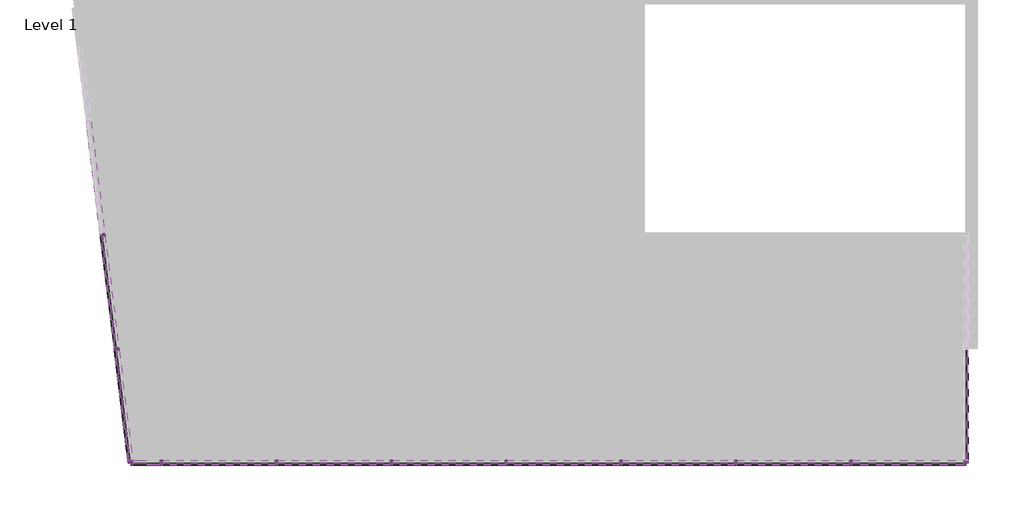
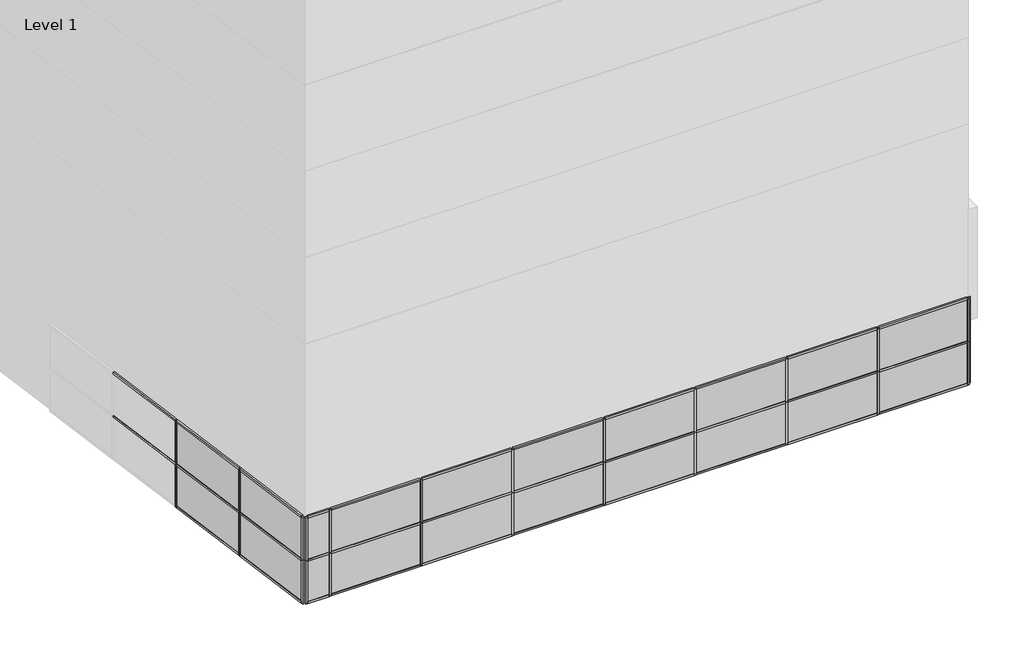
# One storey, part 1 of 2: 60 members, 22 plates.
"""IFC4 building model written with IfcOpenShell, lengths in millimetres."""

from ifc_helpers import new_model, si_unit, origin, place, context, project, spatial, transform, mapped, element, save
from components import member_71c27fd2, member_19d0a4ec, member_8cef0660, member_db480205, member_82905deb, member_4491d118, member_695b83e4, member_0c11e56c, system_panel_glazed_37f15d2e, system_panel_glazed_3620f98e, system_panel_glazed_e46d4b42, system_panel_glazed_2a6c68b7, system_panel_glazed_07b088f8, system_panel_glazed_9d0e0944

model = new_model("IFC4")

# Units and contexts
model_context = context("Model", 3, world=origin())
ifc_project = project(units=[si_unit("LENGTHUNIT", "METRE", prefix="MILLI")], contexts=[model_context])

# Site, building, storey
site = spatial("IfcSite", under=ifc_project)
building = spatial("IfcBuilding", under=site)
storey = spatial("IfcBuildingStorey", under=building, Name="Level 1", Elevation=0.0)

# Members
placement = place(None, origin())
member_shape = member_71c27fd2(model_context)
element("IfcMember", 1, ObjectType="Rectangular Mullion : 2.5\" x 5\" rectangular", at=placement, inside=storey, context=model_context, shape_type="MappedRepresentation", body=[
    mapped(member_shape, transform((-8620.3262186, -3985.3690403, 0.0), x_axis=(0.0, 0.0, -1.0), y_axis=(-0.9925461516413222, -0.12186934340514607, 0.0), z_axis=(-0.12186934340514607, 0.9925461516413222, 0.0))),
])
element("IfcMember", 2, ObjectType="Rectangular Mullion : 2.5\" x 5\" rectangular", at=placement, inside=storey, context=model_context, shape_type="MappedRepresentation", body=[
    mapped(member_shape, transform((10886.265636, -6979.1363705, 0.0), x_axis=(0.0, 0.0, -1.0), y_axis=(0.0, -1.0, 0.0), z_axis=(-1.0, 0.0, 0.0))),
])
element("IfcMember", 3, ObjectType="Rectangular Mullion : 2.5\" x 5\" rectangular", at=placement, inside=storey, context=model_context, shape_type="MappedRepresentation", body=[
    mapped(member_shape, transform((13902.5156363, -6915.6363705, 0.0), x_axis=(0.0, 0.0, -1.0), y_axis=(1.0, 0.0, 0.0), z_axis=(0.0, -1.0, 0.0))),
])
member_2_shape = member_19d0a4ec(model_context)
element("IfcMember", 4, ObjectType="Rectangular Mullion : 2.5\" x 5\" rectangular", at=placement, inside=storey, context=model_context, shape_type="MappedRepresentation", body=[
    mapped(member_2_shape, transform((-8260.4765148, -6916.1096898, 1524.0), x_axis=(0.0, 0.0, 1.0), y_axis=(-0.9925461516413222, -0.12186934340514587, 0.0), z_axis=(0.12186934340514587, -0.9925461516413222, 0.0))),
])
element("IfcMember", 5, ObjectType="Rectangular Mullion : 2.5\" x 5\" rectangular", at=placement, inside=storey, context=model_context, shape_type="MappedRepresentation", body=[
    mapped(member_2_shape, transform((-8260.4765148, -6916.1096898, 3048.0), x_axis=(0.0, 0.0, 1.0), y_axis=(-0.9925461516413222, -0.12186934340514587, 0.0), z_axis=(0.12186934340514587, -0.9925461516413222, 0.0))),
])
element("IfcMember", 6, ObjectType="Rectangular Mullion : 2.5\" x 5\" rectangular", at=placement, inside=storey, context=model_context, shape_type="MappedRepresentation", body=[
    mapped(member_2_shape, transform((13839.0156363, -6979.1363705, 1524.0), x_axis=(0.0, 0.0, 1.0), y_axis=(0.0, -1.0, 0.0), z_axis=(1.0, 0.0, 0.0))),
])
element("IfcMember", 7, ObjectType="Rectangular Mullion : 2.5\" x 5\" rectangular", at=placement, inside=storey, context=model_context, shape_type="MappedRepresentation", body=[
    mapped(member_2_shape, transform((13839.0156363, -6979.1363705, 3048.0), x_axis=(0.0, 0.0, 1.0), y_axis=(0.0, -1.0, 0.0), z_axis=(1.0, 0.0, 0.0))),
])
element("IfcMember", 8, ObjectType="Rectangular Mullion : 2.5\" x 5\" rectangular", at=placement, inside=storey, context=model_context, shape_type="MappedRepresentation", body=[
    mapped(member_2_shape, transform((13902.5156363, -3962.8863708, 1524.0), x_axis=(0.0, 0.0, 1.0), y_axis=(1.0, 0.0, 0.0), z_axis=(0.0, 1.0, 0.0))),
])
member_3_shape = member_8cef0660(model_context)
element("IfcMember", 9, ObjectType="Rectangular Mullion : 2.5\" x 5\" rectangular", at=placement, inside=storey, context=model_context, shape_type="MappedRepresentation", body=[
    mapped(member_3_shape, transform((-8628.0649219, -3922.3423596, 1524.0), x_axis=(0.0, 0.0, 1.0), y_axis=(-0.9925461516413222, -0.12186934340514596, 0.0), z_axis=(0.12186934340514596, -0.9925461516413222, 0.0))),
])
element("IfcMember", 10, ObjectType="Rectangular Mullion : 2.5\" x 5\" rectangular", at=placement, inside=storey, context=model_context, shape_type="MappedRepresentation", body=[
    mapped(member_3_shape, transform((-8999.5226806, -897.0616894, 1524.0), x_axis=(0.0, 0.0, 1.0), y_axis=(-0.9925461516413222, -0.12186934340514566, 0.0), z_axis=(0.12186934340514566, -0.9925461516413222, 0.0))),
])
element("IfcMember", 11, ObjectType="Rectangular Mullion : 2.5\" x 5\" rectangular", at=placement, inside=storey, context=model_context, shape_type="MappedRepresentation", body=[
    mapped(member_3_shape, transform((-8628.0649219, -3922.3423596, 3048.0), x_axis=(0.0, 0.0, 1.0), y_axis=(-0.9925461516413222, -0.12186934340514596, 0.0), z_axis=(0.12186934340514596, -0.9925461516413222, 0.0))),
])
element("IfcMember", 12, ObjectType="Rectangular Mullion : 2.5\" x 5\" rectangular", at=placement, inside=storey, context=model_context, shape_type="MappedRepresentation", body=[
    mapped(member_3_shape, transform((-8999.5226806, -897.0616894, 3048.0), x_axis=(0.0, 0.0, 1.0), y_axis=(-0.9925461516413222, -0.12186934340514602, 0.0), z_axis=(0.12186934340514602, -0.9925461516413222, 0.0))),
])
element("IfcMember", 13, ObjectType="Rectangular Mullion : 2.5\" x 5\" rectangular", at=placement, inside=storey, context=model_context, shape_type="MappedRepresentation", body=[
    mapped(member_3_shape, transform((10822.765636, -6979.1363705, 1524.0), x_axis=(0.0, 0.0, 1.0), y_axis=(0.0, -1.0, 0.0), z_axis=(1.0, 0.0, 0.0))),
])
element("IfcMember", 14, ObjectType="Rectangular Mullion : 2.5\" x 5\" rectangular", at=placement, inside=storey, context=model_context, shape_type="MappedRepresentation", body=[
    mapped(member_3_shape, transform((7774.765636, -6979.1363705, 1524.0), x_axis=(0.0, 0.0, 1.0), y_axis=(0.0, -1.0, 0.0), z_axis=(1.0, 0.0, 0.0))),
])
element("IfcMember", 15, ObjectType="Rectangular Mullion : 2.5\" x 5\" rectangular", at=placement, inside=storey, context=model_context, shape_type="MappedRepresentation", body=[
    mapped(member_3_shape, transform((4726.765636, -6979.1363705, 1524.0), x_axis=(0.0, 0.0, 1.0), y_axis=(0.0, -1.0, 0.0), z_axis=(1.0, 0.0, 0.0))),
])
element("IfcMember", 16, ObjectType="Rectangular Mullion : 2.5\" x 5\" rectangular", at=placement, inside=storey, context=model_context, shape_type="MappedRepresentation", body=[
    mapped(member_3_shape, transform((1678.765636, -6979.1363705, 1524.0), x_axis=(0.0, 0.0, 1.0), y_axis=(0.0, -1.0, 0.0), z_axis=(1.0, 0.0, 0.0))),
])
element("IfcMember", 17, ObjectType="Rectangular Mullion : 2.5\" x 5\" rectangular", at=placement, inside=storey, context=model_context, shape_type="MappedRepresentation", body=[
    mapped(member_3_shape, transform((-1369.234364, -6979.1363705, 1524.0), x_axis=(0.0, 0.0, 1.0), y_axis=(0.0, -1.0, 0.0), z_axis=(1.0, 0.0, 0.0))),
])
element("IfcMember", 18, ObjectType="Rectangular Mullion : 2.5\" x 5\" rectangular", at=placement, inside=storey, context=model_context, shape_type="MappedRepresentation", body=[
    mapped(member_3_shape, transform((-4417.234364, -6979.1363705, 1524.0), x_axis=(0.0, 0.0, 1.0), y_axis=(0.0, -1.0, 0.0), z_axis=(1.0, 0.0, 0.0))),
])
element("IfcMember", 19, ObjectType="Rectangular Mullion : 2.5\" x 5\" rectangular", at=placement, inside=storey, context=model_context, shape_type="MappedRepresentation", body=[
    mapped(member_3_shape, transform((10822.765636, -6979.1363705, 3048.0), x_axis=(0.0, 0.0, 1.0), y_axis=(0.0, -1.0, 0.0), z_axis=(1.0, 0.0, 0.0))),
])
element("IfcMember", 20, ObjectType="Rectangular Mullion : 2.5\" x 5\" rectangular", at=placement, inside=storey, context=model_context, shape_type="MappedRepresentation", body=[
    mapped(member_3_shape, transform((7774.765636, -6979.1363705, 3048.0), x_axis=(0.0, 0.0, 1.0), y_axis=(0.0, -1.0, 0.0), z_axis=(1.0, 0.0, 0.0))),
])
element("IfcMember", 21, ObjectType="Rectangular Mullion : 2.5\" x 5\" rectangular", at=placement, inside=storey, context=model_context, shape_type="MappedRepresentation", body=[
    mapped(member_3_shape, transform((4726.765636, -6979.1363705, 3048.0), x_axis=(0.0, 0.0, 1.0), y_axis=(0.0, -1.0, 0.0), z_axis=(1.0, 0.0, 0.0))),
])
element("IfcMember", 22, ObjectType="Rectangular Mullion : 2.5\" x 5\" rectangular", at=placement, inside=storey, context=model_context, shape_type="MappedRepresentation", body=[
    mapped(member_3_shape, transform((1678.765636, -6979.1363705, 3048.0), x_axis=(0.0, 0.0, 1.0), y_axis=(0.0, -1.0, 0.0), z_axis=(1.0, 0.0, 0.0))),
])
element("IfcMember", 23, ObjectType="Rectangular Mullion : 2.5\" x 5\" rectangular", at=placement, inside=storey, context=model_context, shape_type="MappedRepresentation", body=[
    mapped(member_3_shape, transform((-1369.234364, -6979.1363705, 3048.0), x_axis=(0.0, 0.0, 1.0), y_axis=(0.0, -1.0, 0.0), z_axis=(1.0, 0.0, 0.0))),
])
element("IfcMember", 24, ObjectType="Rectangular Mullion : 2.5\" x 5\" rectangular", at=placement, inside=storey, context=model_context, shape_type="MappedRepresentation", body=[
    mapped(member_3_shape, transform((-4417.234364, -6979.1363705, 3048.0), x_axis=(0.0, 0.0, 1.0), y_axis=(0.0, -1.0, 0.0), z_axis=(1.0, 0.0, 0.0))),
])
member_4_shape = member_db480205(model_context)
element("IfcMember", 25, ObjectType="Rectangular Mullion : 2.5\" x 5\" rectangular", at=placement, inside=storey, context=model_context, shape_type="MappedRepresentation", body=[
    mapped(member_4_shape, transform((-8991.7839773, -960.0883701, 0.0), x_axis=(0.0, 0.0, -1.0), y_axis=(-0.9925461516413222, -0.12186934340514596, 0.0), z_axis=(-0.12186934340514596, 0.9925461516413222, 0.0))),
])
element("IfcMember", 26, ObjectType="Rectangular Mullion : 2.5\" x 5\" rectangular", at=placement, inside=storey, context=model_context, shape_type="MappedRepresentation", body=[
    mapped(member_4_shape, transform((7838.265636, -6979.1363705, 0.0), x_axis=(0.0, 0.0, -1.0), y_axis=(0.0, -1.0, 0.0), z_axis=(-1.0, 0.0, 0.0))),
])
element("IfcMember", 27, ObjectType="Rectangular Mullion : 2.5\" x 5\" rectangular", at=placement, inside=storey, context=model_context, shape_type="MappedRepresentation", body=[
    mapped(member_4_shape, transform((4790.265636, -6979.1363705, 0.0), x_axis=(0.0, 0.0, -1.0), y_axis=(0.0, -1.0, 0.0), z_axis=(-1.0, 0.0, 0.0))),
])
element("IfcMember", 28, ObjectType="Rectangular Mullion : 2.5\" x 5\" rectangular", at=placement, inside=storey, context=model_context, shape_type="MappedRepresentation", body=[
    mapped(member_4_shape, transform((1742.265636, -6979.1363705, 0.0), x_axis=(0.0, 0.0, -1.0), y_axis=(0.0, -1.0, 0.0), z_axis=(-1.0, 0.0, 0.0))),
])
element("IfcMember", 29, ObjectType="Rectangular Mullion : 2.5\" x 5\" rectangular", at=placement, inside=storey, context=model_context, shape_type="MappedRepresentation", body=[
    mapped(member_4_shape, transform((-1305.734364, -6979.1363705, 0.0), x_axis=(0.0, 0.0, -1.0), y_axis=(0.0, -1.0, 0.0), z_axis=(-1.0, 0.0, 0.0))),
])
element("IfcMember", 30, ObjectType="Rectangular Mullion : 2.5\" x 5\" rectangular", at=placement, inside=storey, context=model_context, shape_type="MappedRepresentation", body=[
    mapped(member_4_shape, transform((-4353.734364, -6979.1363705, 0.0), x_axis=(0.0, 0.0, -1.0), y_axis=(0.0, -1.0, 0.0), z_axis=(-1.0, 0.0, 0.0))),
])
element("IfcMember", 31, ObjectType="Rectangular Mullion : 2.5\" x 5\" rectangular", at=placement, inside=storey, context=model_context, shape_type="MappedRepresentation", body=[
    mapped(member_4_shape, transform((-7401.734364, -6979.1363705, 0.0), x_axis=(0.0, 0.0, -1.0), y_axis=(0.0, -1.0, 0.0), z_axis=(-1.0, 0.0, 0.0))),
])
member_5_shape = member_82905deb(model_context)
element("IfcMember", 32, ObjectType="Rectangular Mullion : 2.5\" x 5\" rectangular", at=placement, inside=storey, context=model_context, shape_type="MappedRepresentation", body=[
    mapped(member_5_shape, transform((-8624.1955702, -3953.8557, 1524.0), x_axis=(-0.12186934340514591, 0.9925461516413222, 0.0), y_axis=(-0.9925461516413222, -0.12186934340514591, 0.0), z_axis=(0.0, 0.0, 1.0))),
])
element("IfcMember", 33, ObjectType="Rectangular Mullion : 2.5\" x 5\" rectangular", at=placement, inside=storey, context=model_context, shape_type="MappedRepresentation", body=[
    mapped(member_5_shape, transform((-8995.6533289, -928.5750297, 1524.0), x_axis=(-0.12186934340514591, 0.9925461516413222, 0.0), y_axis=(-0.9925461516413222, -0.12186934340514591, 0.0), z_axis=(0.0, 0.0, 1.0))),
])
element("IfcMember", 34, ObjectType="Rectangular Mullion : 2.5\" x 5\" rectangular", at=placement, inside=storey, context=model_context, shape_type="MappedRepresentation", body=[
    mapped(member_5_shape, transform((10854.515636, -6979.1363705, 1524.0), x_axis=(-1.0, 0.0, 0.0), y_axis=(0.0, -1.0, 0.0), z_axis=(0.0, 0.0, 1.0))),
])
element("IfcMember", 35, ObjectType="Rectangular Mullion : 2.5\" x 5\" rectangular", at=placement, inside=storey, context=model_context, shape_type="MappedRepresentation", body=[
    mapped(member_5_shape, transform((7806.515636, -6979.1363705, 1524.0), x_axis=(-1.0, 0.0, 0.0), y_axis=(0.0, -1.0, 0.0), z_axis=(0.0, 0.0, 1.0))),
])
element("IfcMember", 36, ObjectType="Rectangular Mullion : 2.5\" x 5\" rectangular", at=placement, inside=storey, context=model_context, shape_type="MappedRepresentation", body=[
    mapped(member_5_shape, transform((4758.515636, -6979.1363705, 1524.0), x_axis=(-1.0, 0.0, 0.0), y_axis=(0.0, -1.0, 0.0), z_axis=(0.0, 0.0, 1.0))),
])
element("IfcMember", 37, ObjectType="Rectangular Mullion : 2.5\" x 5\" rectangular", at=placement, inside=storey, context=model_context, shape_type="MappedRepresentation", body=[
    mapped(member_5_shape, transform((1710.515636, -6979.1363705, 1524.0), x_axis=(-1.0, 0.0, 0.0), y_axis=(0.0, -1.0, 0.0), z_axis=(0.0, 0.0, 1.0))),
])
element("IfcMember", 38, ObjectType="Rectangular Mullion : 2.5\" x 5\" rectangular", at=placement, inside=storey, context=model_context, shape_type="MappedRepresentation", body=[
    mapped(member_5_shape, transform((-1337.484364, -6979.1363705, 1524.0), x_axis=(-1.0, 0.0, 0.0), y_axis=(0.0, -1.0, 0.0), z_axis=(0.0, 0.0, 1.0))),
])
element("IfcMember", 39, ObjectType="Rectangular Mullion : 2.5\" x 5\" rectangular", at=placement, inside=storey, context=model_context, shape_type="MappedRepresentation", body=[
    mapped(member_5_shape, transform((-4385.484364, -6979.1363705, 1524.0), x_axis=(-1.0, 0.0, 0.0), y_axis=(0.0, -1.0, 0.0), z_axis=(0.0, 0.0, 1.0))),
])
element("IfcMember", 40, ObjectType="Rectangular Mullion : 2.5\" x 5\" rectangular", at=placement, inside=storey, context=model_context, shape_type="MappedRepresentation", body=[
    mapped(member_5_shape, transform((-7433.484364, -6979.1363705, 1524.0), x_axis=(-1.0, 0.0, 0.0), y_axis=(0.0, -1.0, 0.0), z_axis=(0.0, 0.0, 1.0))),
])
element("IfcMember", 41, ObjectType="Rectangular Mullion : 2.5\" x 5\" rectangular", at=placement, inside=storey, context=model_context, shape_type="MappedRepresentation", body=[
    mapped(member_5_shape, transform((-8624.1955702, -3953.8557, 3048.0), x_axis=(-0.12186934340514591, 0.9925461516413222, 0.0), y_axis=(-0.9925461516413222, -0.12186934340514591, 0.0), z_axis=(0.0, 0.0, 1.0))),
])
element("IfcMember", 42, ObjectType="Rectangular Mullion : 2.5\" x 5\" rectangular", at=placement, inside=storey, context=model_context, shape_type="MappedRepresentation", body=[
    mapped(member_5_shape, transform((-8995.6533289, -928.5750297, 3048.0), x_axis=(-0.12186934340514591, 0.9925461516413222, 0.0), y_axis=(-0.9925461516413222, -0.12186934340514591, 0.0), z_axis=(0.0, 0.0, 1.0))),
])
element("IfcMember", 43, ObjectType="Rectangular Mullion : 2.5\" x 5\" rectangular", at=placement, inside=storey, context=model_context, shape_type="MappedRepresentation", body=[
    mapped(member_5_shape, transform((10854.515636, -6979.1363705, 3048.0), x_axis=(-1.0, 0.0, 0.0), y_axis=(0.0, -1.0, 0.0), z_axis=(0.0, 0.0, 1.0))),
])
element("IfcMember", 44, ObjectType="Rectangular Mullion : 2.5\" x 5\" rectangular", at=placement, inside=storey, context=model_context, shape_type="MappedRepresentation", body=[
    mapped(member_5_shape, transform((7806.515636, -6979.1363705, 3048.0), x_axis=(-1.0, 0.0, 0.0), y_axis=(0.0, -1.0, 0.0), z_axis=(0.0, 0.0, 1.0))),
])
element("IfcMember", 45, ObjectType="Rectangular Mullion : 2.5\" x 5\" rectangular", at=placement, inside=storey, context=model_context, shape_type="MappedRepresentation", body=[
    mapped(member_5_shape, transform((4758.515636, -6979.1363705, 3048.0), x_axis=(-1.0, 0.0, 0.0), y_axis=(0.0, -1.0, 0.0), z_axis=(0.0, 0.0, 1.0))),
])
element("IfcMember", 46, ObjectType="Rectangular Mullion : 2.5\" x 5\" rectangular", at=placement, inside=storey, context=model_context, shape_type="MappedRepresentation", body=[
    mapped(member_5_shape, transform((1710.515636, -6979.1363705, 3048.0), x_axis=(-1.0, 0.0, 0.0), y_axis=(0.0, -1.0, 0.0), z_axis=(0.0, 0.0, 1.0))),
])
element("IfcMember", 47, ObjectType="Rectangular Mullion : 2.5\" x 5\" rectangular", at=placement, inside=storey, context=model_context, shape_type="MappedRepresentation", body=[
    mapped(member_5_shape, transform((-1337.484364, -6979.1363705, 3048.0), x_axis=(-1.0, 0.0, 0.0), y_axis=(0.0, -1.0, 0.0), z_axis=(0.0, 0.0, 1.0))),
])
element("IfcMember", 48, ObjectType="Rectangular Mullion : 2.5\" x 5\" rectangular", at=placement, inside=storey, context=model_context, shape_type="MappedRepresentation", body=[
    mapped(member_5_shape, transform((-4385.484364, -6979.1363705, 3048.0), x_axis=(-1.0, 0.0, 0.0), y_axis=(0.0, -1.0, 0.0), z_axis=(0.0, 0.0, 1.0))),
])
element("IfcMember", 49, ObjectType="Rectangular Mullion : 2.5\" x 5\" rectangular", at=placement, inside=storey, context=model_context, shape_type="MappedRepresentation", body=[
    mapped(member_5_shape, transform((-7433.484364, -6979.1363705, 3048.0), x_axis=(-1.0, 0.0, 0.0), y_axis=(0.0, -1.0, 0.0), z_axis=(0.0, 0.0, 1.0))),
])
member_6_shape = member_4491d118(model_context)
element("IfcMember", 50, ObjectType="Rectangular Mullion : 2.5\" x 5\" rectangular", at=placement, inside=storey, context=model_context, shape_type="MappedRepresentation", body=[
    mapped(member_6_shape, transform((-8252.7378115, -6979.1363705, 0.0), x_axis=(0.12186934340514591, -0.9925461516413222, 0.0), y_axis=(-0.9925461516413222, -0.12186934340514591, 0.0), z_axis=(0.0, 0.0, -1.0))),
])
element("IfcMember", 51, ObjectType="Rectangular Mullion : 2.5\" x 5\" rectangular", at=placement, inside=storey, context=model_context, shape_type="MappedRepresentation", body=[
    mapped(member_6_shape, transform((13902.5156363, -6979.1363705, 0.0), x_axis=(1.0, 0.0, 0.0), y_axis=(0.0, -1.0, 0.0), z_axis=(0.0, 0.0, -1.0))),
])
element("IfcMember", 52, ObjectType="Rectangular Mullion : 2.5\" x 5\" rectangular", at=placement, inside=storey, context=model_context, shape_type="MappedRepresentation", body=[
    mapped(member_6_shape, transform((-8252.7378115, -6979.1363705, 1524.0), x_axis=(0.12186934340514591, -0.9925461516413222, 0.0), y_axis=(-0.9925461516413222, -0.12186934340514591, 0.0), z_axis=(0.0, 0.0, -1.0))),
])
element("IfcMember", 53, ObjectType="Rectangular Mullion : 2.5\" x 5\" rectangular", at=placement, inside=storey, context=model_context, shape_type="MappedRepresentation", body=[
    mapped(member_6_shape, transform((13902.5156363, -6979.1363705, 1524.0), x_axis=(1.0, 0.0, 0.0), y_axis=(0.0, -1.0, 0.0), z_axis=(0.0, 0.0, -1.0))),
])
element("IfcMember", 54, ObjectType="Rectangular Mullion : 2.5\" x 5\" rectangular", at=placement, inside=storey, context=model_context, shape_type="MappedRepresentation", body=[
    mapped(member_6_shape, transform((-8252.7378115, -6979.1363705, 1524.0), x_axis=(-1.0, 0.0, 0.0), y_axis=(0.0, -1.0, 0.0), z_axis=(0.0, 0.0, 1.0))),
])
element("IfcMember", 55, ObjectType="Rectangular Mullion : 2.5\" x 5\" rectangular", at=placement, inside=storey, context=model_context, shape_type="MappedRepresentation", body=[
    mapped(member_6_shape, transform((13902.5156363, -6979.1363705, 1524.0), x_axis=(0.0, -1.0, 0.0), y_axis=(1.0, 0.0, 0.0), z_axis=(0.0, 0.0, 1.0))),
])
element("IfcMember", 56, ObjectType="Rectangular Mullion : 2.5\" x 5\" rectangular", at=placement, inside=storey, context=model_context, shape_type="MappedRepresentation", body=[
    mapped(member_6_shape, transform((-8252.7378115, -6979.1363705, 3048.0), x_axis=(-1.0, 0.0, 0.0), y_axis=(0.0, -1.0, 0.0), z_axis=(0.0, 0.0, 1.0))),
])
element("IfcMember", 57, ObjectType="Rectangular Mullion : 2.5\" x 5\" rectangular", at=placement, inside=storey, context=model_context, shape_type="MappedRepresentation", body=[
    mapped(member_6_shape, transform((13902.5156363, -6979.1363705, 3048.0), x_axis=(0.0, -1.0, 0.0), y_axis=(1.0, 0.0, 0.0), z_axis=(0.0, 0.0, 1.0))),
])
member_7_shape = member_695b83e4(model_context)
element("IfcMember", 58, ObjectType="Rectangular Mullion : 2.5\" x 5\" rectangular", at=placement, inside=storey, context=model_context, shape_type="MappedRepresentation", body=[
    mapped(member_7_shape, transform((-8189.2378115, -6979.1363705, 0.0), x_axis=(0.0, 0.0, -1.0), y_axis=(0.0, -1.0, 0.0), z_axis=(-1.0, 0.0, 0.0))),
])
member_8_shape = member_0c11e56c(model_context)
element("IfcMember", 59, ObjectType="Rectangular Mullion : 2.5\" x 5\" rectangular", at=placement, inside=storey, context=model_context, shape_type="MappedRepresentation", body=[
    mapped(member_8_shape, transform((-7465.234364, -6979.1363705, 1524.0), x_axis=(0.0, 0.0, 1.0), y_axis=(0.0, -1.0, 0.0), z_axis=(1.0, 0.0, 0.0))),
])
element("IfcMember", 60, ObjectType="Rectangular Mullion : 2.5\" x 5\" rectangular", at=placement, inside=storey, context=model_context, shape_type="MappedRepresentation", body=[
    mapped(member_8_shape, transform((-7465.234364, -6979.1363705, 3048.0), x_axis=(0.0, 0.0, 1.0), y_axis=(0.0, -1.0, 0.0), z_axis=(1.0, 0.0, 0.0))),
])

# Plates
system_panel_glazed_shape = system_panel_glazed_37f15d2e(model_context)
element("IfcPlate", 61, ObjectType="System Panel : Glazed", at=placement, inside=storey, context=model_context, shape_type="MappedRepresentation", body=[
    mapped(system_panel_glazed_shape, transform((-8440.4013667, -5450.739365, 63.5), x_axis=(-0.12186934340514591, 0.9925461516413222, 0.0), y_axis=(-0.9925461516413222, -0.12186934340514591, 0.0), z_axis=(0.0, 0.0, 1.0))),
])
element("IfcPlate", 62, ObjectType="System Panel : Glazed", at=placement, inside=storey, context=model_context, shape_type="MappedRepresentation", body=[
    mapped(system_panel_glazed_shape, transform((12362.6406361, -6979.1363705, 63.5), x_axis=(-1.0, 0.0, 0.0), y_axis=(0.0, -1.0, 0.0), z_axis=(0.0, 0.0, 1.0))),
])
element("IfcPlate", 63, ObjectType="System Panel : Glazed", at=placement, inside=storey, context=model_context, shape_type="MappedRepresentation", body=[
    mapped(system_panel_glazed_shape, transform((13902.5156363, -5439.2613706, 63.5), x_axis=(0.0, -1.0, 0.0), y_axis=(1.0, 0.0, 0.0), z_axis=(0.0, 0.0, 1.0))),
])
system_panel_glazed_2_shape = system_panel_glazed_3620f98e(model_context)
element("IfcPlate", 64, ObjectType="System Panel : Glazed", at=placement, inside=storey, context=model_context, shape_type="MappedRepresentation", body=[
    mapped(system_panel_glazed_2_shape, transform((-8809.9244496, -2441.2153649, 63.5), x_axis=(-0.12186934340514591, 0.9925461516413222, 0.0), y_axis=(-0.9925461516413222, -0.12186934340514591, 0.0), z_axis=(0.0, 0.0, 1.0))),
])
element("IfcPlate", 65, ObjectType="System Panel : Glazed", at=placement, inside=storey, context=model_context, shape_type="MappedRepresentation", body=[
    mapped(system_panel_glazed_2_shape, transform((9330.515636, -6979.1363705, 63.5), x_axis=(-1.0, 0.0, 0.0), y_axis=(0.0, -1.0, 0.0), z_axis=(0.0, 0.0, 1.0))),
])
element("IfcPlate", 66, ObjectType="System Panel : Glazed", at=placement, inside=storey, context=model_context, shape_type="MappedRepresentation", body=[
    mapped(system_panel_glazed_2_shape, transform((6282.515636, -6979.1363705, 63.5), x_axis=(-1.0, 0.0, 0.0), y_axis=(0.0, -1.0, 0.0), z_axis=(0.0, 0.0, 1.0))),
])
element("IfcPlate", 67, ObjectType="System Panel : Glazed", at=placement, inside=storey, context=model_context, shape_type="MappedRepresentation", body=[
    mapped(system_panel_glazed_2_shape, transform((3234.515636, -6979.1363705, 63.5), x_axis=(-1.0, 0.0, 0.0), y_axis=(0.0, -1.0, 0.0), z_axis=(0.0, 0.0, 1.0))),
])
element("IfcPlate", 68, ObjectType="System Panel : Glazed", at=placement, inside=storey, context=model_context, shape_type="MappedRepresentation", body=[
    mapped(system_panel_glazed_2_shape, transform((186.515636, -6979.1363705, 63.5), x_axis=(-1.0, 0.0, 0.0), y_axis=(0.0, -1.0, 0.0), z_axis=(0.0, 0.0, 1.0))),
])
element("IfcPlate", 69, ObjectType="System Panel : Glazed", at=placement, inside=storey, context=model_context, shape_type="MappedRepresentation", body=[
    mapped(system_panel_glazed_2_shape, transform((-2861.484364, -6979.1363705, 63.5), x_axis=(-1.0, 0.0, 0.0), y_axis=(0.0, -1.0, 0.0), z_axis=(0.0, 0.0, 1.0))),
])
element("IfcPlate", 70, ObjectType="System Panel : Glazed", at=placement, inside=storey, context=model_context, shape_type="MappedRepresentation", body=[
    mapped(system_panel_glazed_2_shape, transform((-5909.484364, -6979.1363705, 63.5), x_axis=(-1.0, 0.0, 0.0), y_axis=(0.0, -1.0, 0.0), z_axis=(0.0, 0.0, 1.0))),
])
system_panel_glazed_3_shape = system_panel_glazed_e46d4b42(model_context)
element("IfcPlate", 71, ObjectType="System Panel : Glazed", at=placement, inside=storey, context=model_context, shape_type="MappedRepresentation", body=[
    mapped(system_panel_glazed_3_shape, transform((-8440.4013667, -5450.739365, 1555.75), x_axis=(-0.12186934340514591, 0.9925461516413222, 0.0), y_axis=(-0.9925461516413222, -0.12186934340514591, 0.0), z_axis=(0.0, 0.0, 1.0))),
])
element("IfcPlate", 72, ObjectType="System Panel : Glazed", at=placement, inside=storey, context=model_context, shape_type="MappedRepresentation", body=[
    mapped(system_panel_glazed_3_shape, transform((12362.6406361, -6979.1363705, 1555.75), x_axis=(-1.0, 0.0, 0.0), y_axis=(0.0, -1.0, 0.0), z_axis=(0.0, 0.0, 1.0))),
])
element("IfcPlate", 73, ObjectType="System Panel : Glazed", at=placement, inside=storey, context=model_context, shape_type="MappedRepresentation", body=[
    mapped(system_panel_glazed_3_shape, transform((13902.5156363, -5439.2613706, 1555.75), x_axis=(0.0, -1.0, 0.0), y_axis=(1.0, 0.0, 0.0), z_axis=(0.0, 0.0, 1.0))),
])
system_panel_glazed_4_shape = system_panel_glazed_2a6c68b7(model_context)
element("IfcPlate", 74, ObjectType="System Panel : Glazed", at=placement, inside=storey, context=model_context, shape_type="MappedRepresentation", body=[
    mapped(system_panel_glazed_4_shape, transform((-8809.9244496, -2441.2153649, 1555.75), x_axis=(-0.12186934340514591, 0.9925461516413222, 0.0), y_axis=(-0.9925461516413222, -0.12186934340514591, 0.0), z_axis=(0.0, 0.0, 1.0))),
])
element("IfcPlate", 75, ObjectType="System Panel : Glazed", at=placement, inside=storey, context=model_context, shape_type="MappedRepresentation", body=[
    mapped(system_panel_glazed_4_shape, transform((9330.515636, -6979.1363705, 1555.75), x_axis=(-1.0, 0.0, 0.0), y_axis=(0.0, -1.0, 0.0), z_axis=(0.0, 0.0, 1.0))),
])
element("IfcPlate", 76, ObjectType="System Panel : Glazed", at=placement, inside=storey, context=model_context, shape_type="MappedRepresentation", body=[
    mapped(system_panel_glazed_4_shape, transform((6282.515636, -6979.1363705, 1555.75), x_axis=(-1.0, 0.0, 0.0), y_axis=(0.0, -1.0, 0.0), z_axis=(0.0, 0.0, 1.0))),
])
element("IfcPlate", 77, ObjectType="System Panel : Glazed", at=placement, inside=storey, context=model_context, shape_type="MappedRepresentation", body=[
    mapped(system_panel_glazed_4_shape, transform((3234.515636, -6979.1363705, 1555.75), x_axis=(-1.0, 0.0, 0.0), y_axis=(0.0, -1.0, 0.0), z_axis=(0.0, 0.0, 1.0))),
])
element("IfcPlate", 78, ObjectType="System Panel : Glazed", at=placement, inside=storey, context=model_context, shape_type="MappedRepresentation", body=[
    mapped(system_panel_glazed_4_shape, transform((186.515636, -6979.1363705, 1555.75), x_axis=(-1.0, 0.0, 0.0), y_axis=(0.0, -1.0, 0.0), z_axis=(0.0, 0.0, 1.0))),
])
element("IfcPlate", 79, ObjectType="System Panel : Glazed", at=placement, inside=storey, context=model_context, shape_type="MappedRepresentation", body=[
    mapped(system_panel_glazed_4_shape, transform((-2861.484364, -6979.1363705, 1555.75), x_axis=(-1.0, 0.0, 0.0), y_axis=(0.0, -1.0, 0.0), z_axis=(0.0, 0.0, 1.0))),
])
element("IfcPlate", 80, ObjectType="System Panel : Glazed", at=placement, inside=storey, context=model_context, shape_type="MappedRepresentation", body=[
    mapped(system_panel_glazed_4_shape, transform((-5909.484364, -6979.1363705, 1555.75), x_axis=(-1.0, 0.0, 0.0), y_axis=(0.0, -1.0, 0.0), z_axis=(0.0, 0.0, 1.0))),
])
system_panel_glazed_5_shape = system_panel_glazed_07b088f8(model_context)
element("IfcPlate", 81, ObjectType="System Panel : Glazed", at=placement, inside=storey, context=model_context, shape_type="MappedRepresentation", body=[
    mapped(system_panel_glazed_5_shape, transform((-7827.2360878, -6979.1363705, 63.5), x_axis=(-1.0, 0.0, 0.0), y_axis=(0.0, -1.0, 0.0), z_axis=(0.0, 0.0, 1.0))),
])
system_panel_glazed_6_shape = system_panel_glazed_9d0e0944(model_context)
element("IfcPlate", 82, ObjectType="System Panel : Glazed", at=placement, inside=storey, context=model_context, shape_type="MappedRepresentation", body=[
    mapped(system_panel_glazed_6_shape, transform((-7827.2360878, -6979.1363705, 1555.75), x_axis=(-1.0, 0.0, 0.0), y_axis=(0.0, -1.0, 0.0), z_axis=(0.0, 0.0, 1.0))),
])

save(model, "model.ifc")

# Revit data of these elements
# Type "Rectangular Mullion : 2.5\" x 5\" rectangular"
#   built-in parameter 1007304 = 0.416667 (stored number, unit not read)
#   built-in parameter 1007301 = 0.104167 (stored number, unit not read)
#   built-in parameter 1007300 = 0.104167 (stored number, unit not read)
# Type "System Panel : Glazed"
#   Construction Type Id = "GSP4R"
#   Analytic Construction = "1/8 in Pilkington single glazing"
#   Visual Light Transmittance = 0.9
#   Solar Heat Gain Coefficient = 0.86
#   Heat Transfer Coefficient (U) = 1.18115 BTU/(h·ft²·°F)
#   Define Thermal Properties by = 1
# Elements 1, 2, 3, 4, 5, 6, 7, 8, 9, 10, 11, 12, 13, 14, 15, 16, 17, 18, 19, 20, 21, 22, 23, 24, 25, 26, 27, 28, 29, 30, 31, 32, 33, 34, 35, 36, 37, 38, 39, 40, 41, 42, 43, 44, 45, 46, 47, 48, 49, 50, 51, 52, 53, 54, 55, 56, 57, 58, 59, 60 (IfcMember, "Rectangular Mullion : 2.5\" x 5\" rectangular")
#   Phase Created = New Construction
#   Materials on its faces: "Aluminum"
# Elements 61, 62, 63, 64, 65, 66, 67, 68, 69, 70, 71, 72, 73, 74, 75, 76, 77, 78, 79, 80, 81, 82 (IfcPlate, "System Panel : Glazed")
#   Phase Created = New Construction
#   Materials on its faces: "Glass"
# Materials
#   "Aluminum": class "Metal", colour RGB 247 247 247, transparency 0, Description = "Aluminum 6061", Cost = 0
#   "Glass": class "Glass", colour RGB 0 128 192, transparency 0.75, Description = "Soda Lime Glass", Cost = 0
